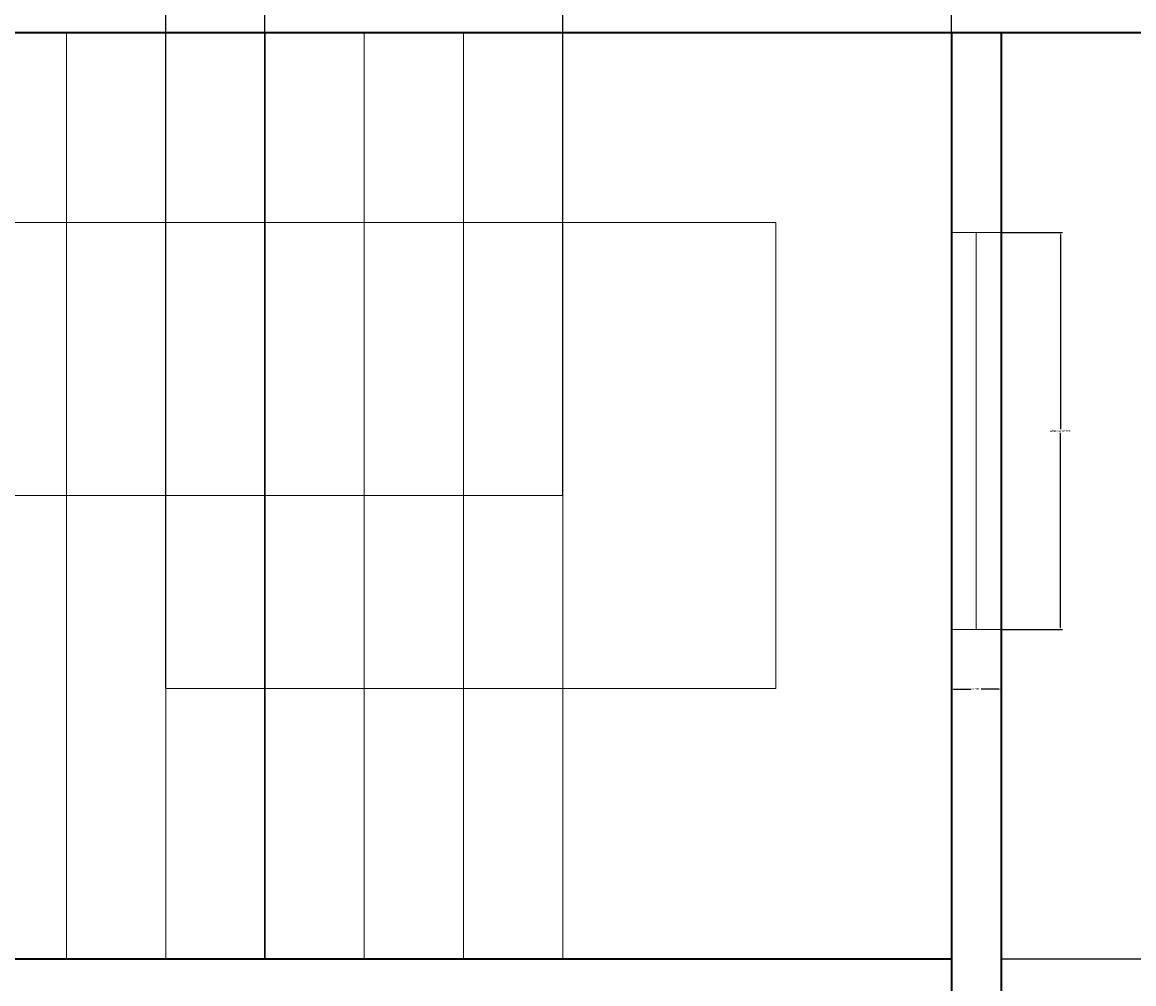
# Model space of a CAD drawing. Units: inches. Extents: x 1088 to 1703, y 668 to 1875.
# Tile 6 of 45: x 1502 to 1602, y 1329 to 1416. Entities that reach past the tile are written whole.
import ezdxf

# ---------------------------------------------------------------- set-up
doc = ezdxf.new("R2010")
doc.units = ezdxf.units.IN
for name, color, linetype, lineweight in [('A-ANNO-DIMS', 2, 'Continuous', 18), ('A-ANNO-SYMB', 7, 'Continuous', 18), ('A-FLOR-HRAL', 7, 'Continuous', 25), ('A-FLOR-STRS', 7, 'Continuous', 18), ('A-GLAZ', 4, 'Continuous', 18), ('A-WALL', 7, 'Continuous', 35)]:
    doc.layers.add(name, color=color, linetype=linetype, lineweight=lineweight)
doc.styles.get("Standard").update_dxf_attribs({"font": 'arial.ttf'})
doc.dimstyles.get("Standard").update_dxf_attribs({"dimtxt": 0.18, "dimasz": 0.18, "dimexe": 0.18, "dimexo": 0.0625, "dimgap": 0.09, "dimtad": 0, "dimtih": 1, "dimtoh": 1, "dimdec": 4, "dimzin": 0, "dimdsep": 46, "dimtxsty": 'Standard', "dimcen": 0.09, "dimadec": 0, "dimazin": 0, "dimtfac": 1, "dimtdec": 4, "dimtofl": 0, "dimtmove": 0, "dimatfit": 3, "dimfxl": 1, "dimtolj": 1, "dimtzin": 0, "dimarcsym": 0})

# ---------------------------------------------------------------- blocks, each defined once
blk = doc.blocks.new('WIN-36-RETURN')
for p, q in [((0, 36), (4.5, 36)), ((4.5, 36), (2.25, 36)), ((2.25, 36), (2.25, 0)), ((4.5, 0), (0, 0)), ((2.25, 0), (4.5, 0))]:
    blk.add_line(p, q)
blk = doc.blocks.new('*D22')
at = {"layer": 'A-ANNO-DIMS', "color": 0, "lineweight": -2, "transparency": 16777216}
for p, q in [((1590.41, 1396.92), (1595.92, 1396.92)), ((1595.74, 1396.74), (1595.74, 1379.1)), ((1595.74, 1361.1), (1595.74, 1378.74)), ((1590.41, 1360.92), (1595.92, 1360.92))]:
    blk.add_line(p, q, dxfattribs=at)
at = {"layer": 'A-ANNO-DIMS', "color": 0, "transparency": 16777216}
for points in [[(1595.71, 1396.74), (1595.77, 1396.74), (1595.74, 1396.92)], [(1595.71, 1361.1), (1595.77, 1361.1), (1595.74, 1360.92)]]:
    blk.add_solid(points, dxfattribs=at)
at = {"layer": 'Defpoints', "color": 0, "transparency": 16777216}
for p in [(1590.34, 1396.92), (1595.74, 1396.92), (1590.34, 1360.92)]:
    blk.add_point(p, dxfattribs=at)
at = {"layer": 'A-ANNO-DIMS', "color": 0, "transparency": 16777216, "insert": (1595.74, 1378.92), "char_height": 0.18, "attachment_point": 5}
blk.add_mtext('\\A1;WINDOW 36 TYP.', dxfattribs=at)
blk = doc.blocks.new('*D23')
at = {"layer": 'A-ANNO-DIMS', "color": 0, "lineweight": -2, "transparency": 16777216}
for p, q in [((1585.84, 1360.86), (1585.84, 1355.34)), ((1590.34, 1360.86), (1590.34, 1355.34)), ((1586.02, 1355.52), (1587.64, 1355.52)), ((1590.16, 1355.52), (1588.55, 1355.52))]:
    blk.add_line(p, q, dxfattribs=at)
at = {"layer": 'A-ANNO-DIMS', "color": 0, "transparency": 16777216}
for points in [[(1586.02, 1355.55), (1586.02, 1355.49), (1585.84, 1355.52)], [(1590.16, 1355.55), (1590.16, 1355.49), (1590.34, 1355.52)]]:
    blk.add_solid(points, dxfattribs=at)
at = {"layer": 'Defpoints', "color": 0, "transparency": 16777216}
for p in [(1585.84, 1360.92), (1590.34, 1360.92), (1590.34, 1355.52)]:
    blk.add_point(p, dxfattribs=at)
at = {"layer": 'A-ANNO-DIMS', "color": 0, "transparency": 16777216, "insert": (1588.09, 1355.52), "char_height": 0.18, "attachment_point": 5}
blk.add_mtext('\\A1;5 TYP.', dxfattribs=at)
blk = doc.blocks.new('*D32')
at = {"layer": 'A-ANNO-DIMS', "color": 0, "lineweight": -2, "transparency": 16777216}
for p, q in [((1550.59, 1373.12), (1550.59, 1857.79)), ((1585.84, 1360.98), (1585.84, 1857.79)), ((1550.77, 1857.61), (1567.83, 1857.61)), ((1585.66, 1857.61), (1568.61, 1857.61))]:
    blk.add_line(p, q, dxfattribs=at)
at = {"layer": 'A-ANNO-DIMS', "color": 0, "transparency": 16777216}
for points in [[(1550.77, 1857.64), (1550.77, 1857.58), (1550.59, 1857.61)], [(1585.66, 1857.64), (1585.66, 1857.58), (1585.84, 1857.61)]]:
    blk.add_solid(points, dxfattribs=at)
at = {"layer": 'Defpoints', "color": 0, "transparency": 16777216}
for p in [(1585.84, 1857.61), (1550.59, 1373.06), (1585.84, 1360.92)]:
    blk.add_point(p, dxfattribs=at)
at = {"layer": 'A-ANNO-DIMS', "color": 0, "transparency": 16777216, "insert": (1568.22, 1857.61), "char_height": 0.18, "attachment_point": 5}
blk.add_mtext('\\A1;35.25', dxfattribs=at)
blk = doc.blocks.new('*D33')
at = {"layer": 'A-ANNO-DIMS', "color": 0, "lineweight": -2, "transparency": 16777216}
for p, q in [((1514.59, 1355.65), (1514.59, 1857.79)), ((1523.59, 1331.12), (1523.59, 1857.79)), ((1514.77, 1857.61), (1518.95, 1857.61)), ((1523.41, 1857.61), (1519.24, 1857.61))]:
    blk.add_line(p, q, dxfattribs=at)
at = {"layer": 'A-ANNO-DIMS', "color": 0, "transparency": 16777216}
for points in [[(1514.77, 1857.64), (1514.77, 1857.58), (1514.59, 1857.61)], [(1523.41, 1857.64), (1523.41, 1857.58), (1523.59, 1857.61)]]:
    blk.add_solid(points, dxfattribs=at)
at = {"layer": 'Defpoints', "color": 0, "transparency": 16777216}
for p in [(1523.59, 1857.61), (1514.59, 1355.59), (1523.59, 1331.06)]:
    blk.add_point(p, dxfattribs=at)
at = {"layer": 'A-ANNO-DIMS', "color": 0, "transparency": 16777216, "insert": (1519.09, 1857.61), "char_height": 0.18, "attachment_point": 5}
blk.add_mtext('\\A1;9', dxfattribs=at)

msp = doc.modelspace()

# ---------------------------------------------------------------- linework, layer by layer
at = {"layer": 'A-ANNO-SYMB'}
for p, q in [((1451.148, 1397.817), (1569.925, 1397.817)), ((1569.925, 1397.817), (1569.925, 1355.585)), ((1569.925, 1355.585), (1514.595, 1355.585))]:
    msp.add_line(p, q, dxfattribs=at)
at = {"layer": 'A-FLOR-HRAL'}
msp.add_line((1590.345, 1331.058), (1642.243, 1331.058), dxfattribs=at)
at = {"layer": 'A-FLOR-STRS'}
for p, q in [((1505.595, 1415.058), (1505.595, 1331.058)), ((1514.595, 1415.058), (1514.595, 1331.058)), ((1523.595, 1415.058), (1523.595, 1331.058)), ((1532.595, 1415.058), (1532.595, 1331.058)), ((1541.595, 1415.058), (1541.595, 1331.058)), ((1550.595, 1415.058), (1550.595, 1331.058)), ((1460.595, 1373.058), (1550.595, 1373.058))]:
    msp.add_line(p, q, dxfattribs=at)
at = {"layer": 'A-WALL'}
for p, q in [((1485.345, 1415.058), (1590.345, 1415.058)), ((1585.845, 1415.058), (1585.845, 1185.558)), ((1590.345, 1415.058), (1614.345, 1415.058)), ((1590.345, 1415.058), (1590.345, 1185.558)), ((1435.845, 1331.058), (1585.845, 1331.058))]:
    msp.add_line(p, q, dxfattribs=at)

# ---------------------------------------------------------------- block references
at = {"layer": 'A-GLAZ'}
msp.add_blockref('WIN-36-RETURN', (1585.845, 1360.921), dxfattribs=at)

# ---------------------------------------------------------------- dimensions: what is measured, and where the dimension line sits
at = {"layer": 'A-ANNO-DIMS'}
for base, p1, p2, override, picture, middle in [((1523.595, 1857.608), (1514.595, 1355.585), (1523.595, 1331.058), {"dimdec": 0, "dimlfac": 1, "dimrnd": 0, "dimzin": 0, "dimdsep": 46, "dimlunit": 2}, '*D33', (1519.095, 1857.608)), ((1585.845, 1857.608), (1550.595, 1373.058), (1585.845, 1360.921), {"dimdec": 2, "dimlfac": 1, "dimrnd": 0, "dimzin": 0, "dimdsep": 46, "dimlunit": 2}, '*D32', (1568.22, 1857.608))]:
    dim = msp.add_linear_dim(base=base, p1=p1, p2=p2, dimstyle='Standard', override=override, dxfattribs=at)
    dim.commit()
    dim.dimension.update_dxf_attribs({"geometry": picture, "text_midpoint": middle})
dim = msp.add_linear_dim(base=(1595.745, 1396.921), p1=(1590.345, 1360.921), p2=(1590.345, 1396.921), angle=90, text='WINDOW <> TYP.', dimstyle='Standard', override={"dimdec": 0, "dimlfac": 1, "dimrnd": 0, "dimzin": 0, "dimdsep": 46, "dimlunit": 2}, dxfattribs=at)
dim.commit()
dim.dimension.update_dxf_attribs({"geometry": '*D22', "text_midpoint": (1595.745, 1378.921)})
dim = msp.add_linear_dim(base=(1590.344800082, 1355.520514812), p1=(1585.844800082, 1360.920514812), p2=(1590.344800082, 1360.920514812), text='<> TYP.', dimstyle='Standard', override={"dimdec": 0, "dimlfac": 1, "dimrnd": 0, "dimzin": 0, "dimdsep": 46, "dimlunit": 2}, dxfattribs=at)
dim.commit()
dim.dimension.update_dxf_attribs({"geometry": '*D23', "text_midpoint": (1588.094800082, 1355.520514812)})

doc.saveas('drawing.dxf')
